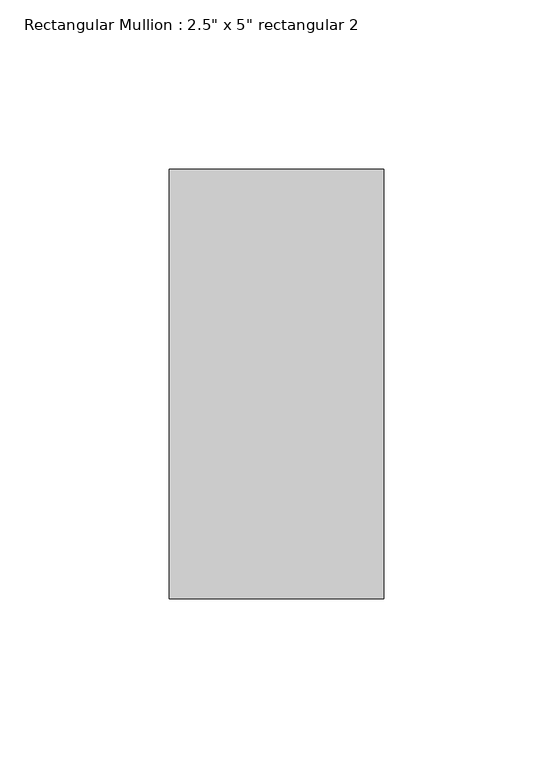
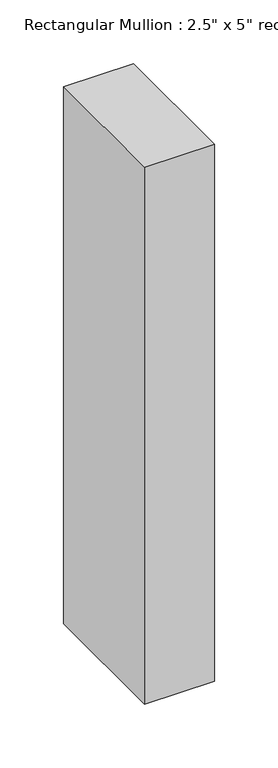
"""IFC4 building model written with IfcOpenShell, lengths in millimetres: member geometry."""

from ifc_helpers import new_model, si_unit, frame, origin, place, context, project, spatial, polyline, outline, extrude, source, transform, mapped, element, save


def member_0b7646a3(model_context):
    return source(origin(), model_context, "Body", "SweptSolid", [
        extrude(outline(polyline([(0.0, 63.5), (0.0, -63.5), (-63.5, -63.5), (-63.5, 63.5), (0.0, 63.5)])), frame((0.0, 0.0, -514.35), z_axis=(0.0, 0.0, 1.0), x_axis=(1.0, 0.0, 0.0)), (0.0, 0.0, 1.0), 514.35),
    ])


if __name__ == "__main__":
    model = new_model("IFC4")
    model_context = context("Model", 3, world=origin())
    ifc_project = project(units=[si_unit("LENGTHUNIT", "METRE", prefix="MILLI")], contexts=[model_context])
    site = spatial("IfcSite", under=ifc_project)
    building = spatial("IfcBuilding", under=site)
    placement = place(None, origin())
    member_shape = member_0b7646a3(model_context)
    element("IfcMember", 1, ObjectType="Rectangular Mullion : 2.5\" x 5\" rectangular 2", at=placement, inside=building, context=model_context, shape_type="MappedRepresentation", body=[
        mapped(member_shape, transform((0.0, 0.0, 0.0), x_axis=(1.0, 0.0, 0.0), y_axis=(0.0, 1.0, 0.0), z_axis=(0.0, 0.0, 1.0))),
    ])
    save(model, "model.ifc")

# Revit data of these elements
# Type "Rectangular Mullion : 2.5\" x 5\" rectangular 2"
#   built-in parameter 1007304 = 0.416667 (stored number, unit not read)
#   built-in parameter 1007301 = 0.104167 (stored number, unit not read)
#   built-in parameter 1007300 = 0.104167 (stored number, unit not read)
